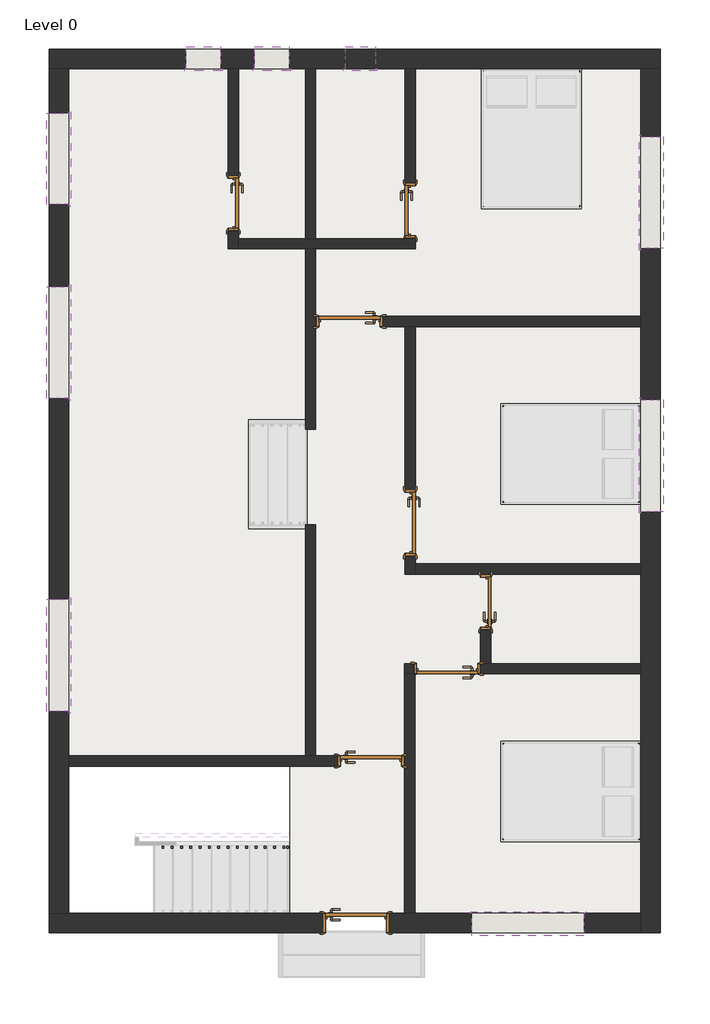
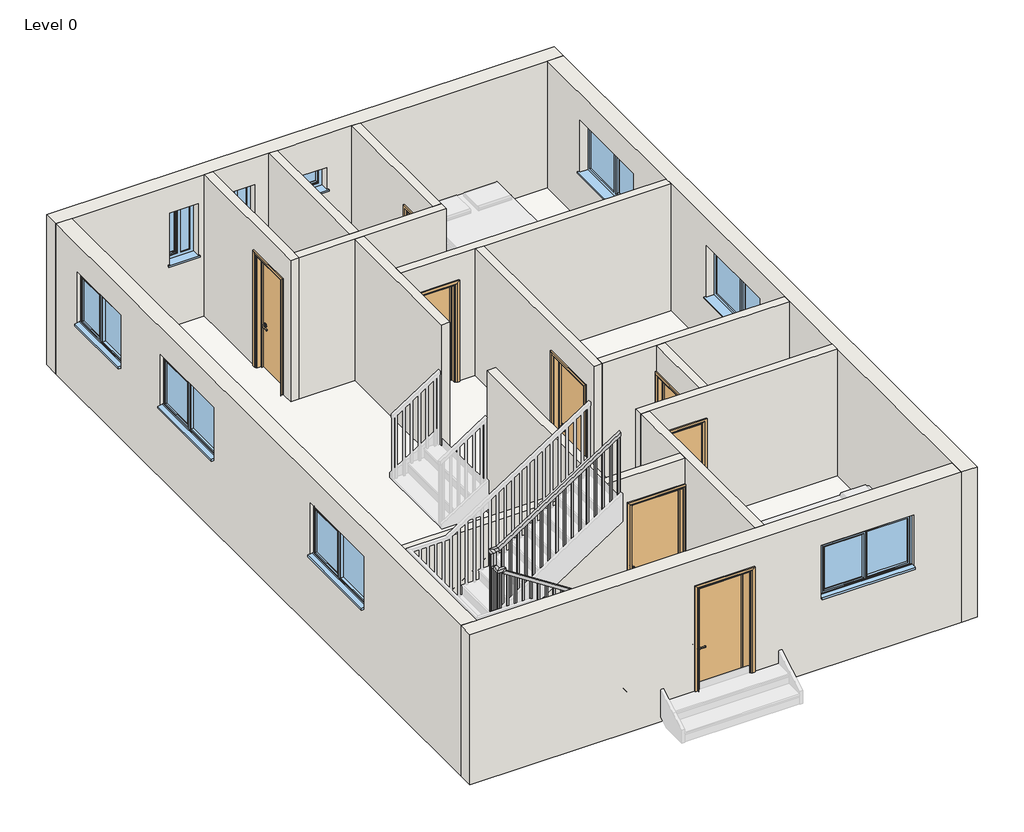
# One storey, part 1 of 2: 16 walls, 9 windows, 8 doors, 2 slabs, 1 railing.
# Revit data of these elements (continued)
# Materials (continued)
#   "Door - Panel": class "Wood", colour RGB 210 159 95, transparency 0, Keynote = "L20", Cost = 0
#   "Door - Architrave": class "Wood", colour RGB 154 90 5, transparency 0, Keynote = "P20", Cost = 0
#   "Wood Sheathing, Chipboard": class "Wood", colour RGB 127 127 127, transparency 0, Description = "Particleboard sheathing", Cost = 0
#   "Structure, Timber Joist/Rafter Layer": class "Wood", colour RGB 127 127 127, transparency 0, Description = "Timber framing, thermal airspace", Cost = 0
#   "Brick, Common": class "Masonry", colour RGB 170 100 105, transparency 0, Description = "Common brick", Cost = 0
#   "Window Frame": colour RGB 249 249 249, transparency 0, Keynote = "L10", Cost = 0
#   "Glass": class "Glass", colour RGB 0 128 192, transparency 0.9, Description = "Soda Lime Glass", Cost = 0
